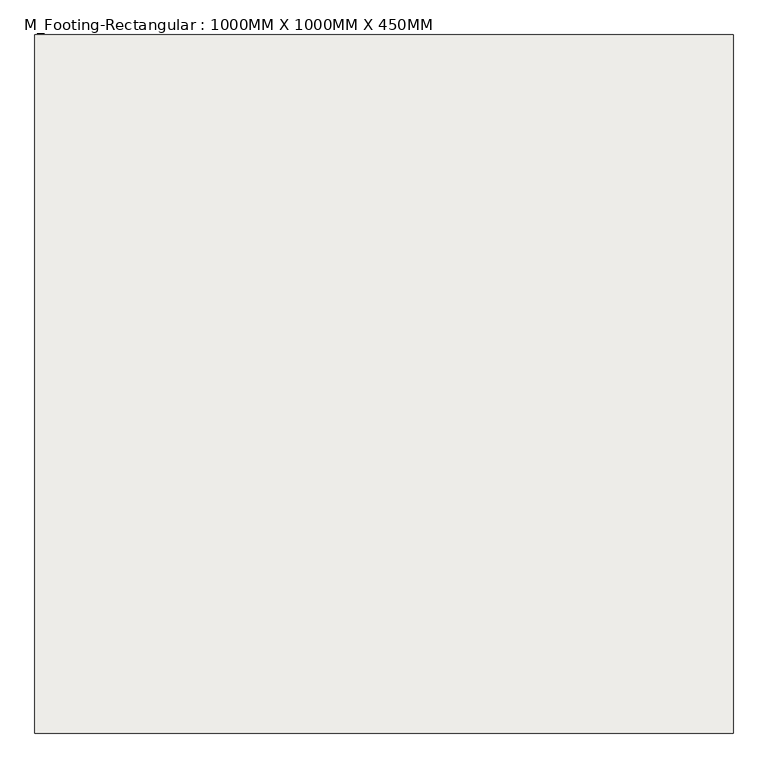
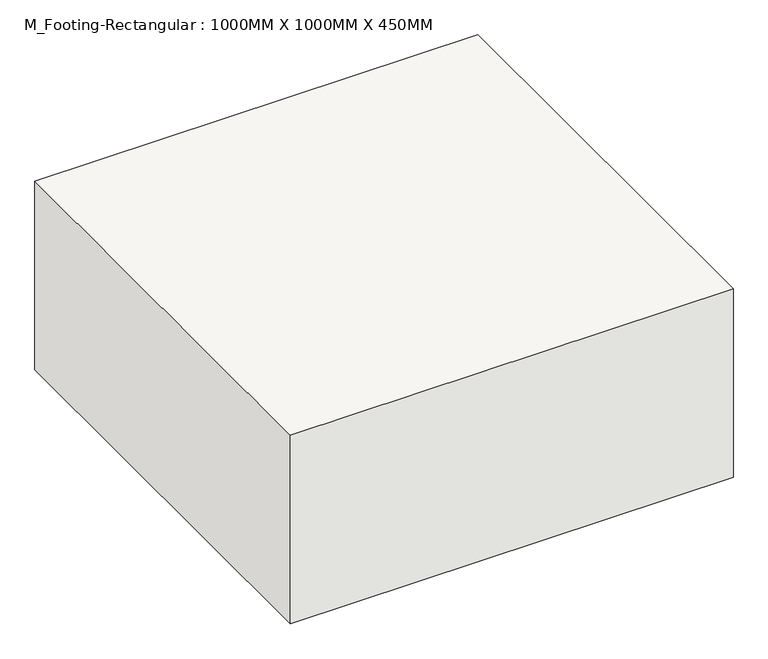
"""IFC4 building model written with IfcOpenShell, lengths in millimetres: slab geometry, M_Footing-Rectangular : 1000MM X 1000MM X 450MM."""

from ifc_helpers import new_model, si_unit, frame, origin, place, context, project, spatial, polyline, outline, extrude, source, transform, mapped, element, save


def m_footing_rectangular_1000mm_x_1000mm_x_450mm_4c97ae35(model_context):
    return source(origin(), model_context, "Body", "SweptSolid", [
        extrude(outline(polyline([(500.0, 500.0), (500.0, -500.0), (-500.0, -500.0), (-500.0, 500.0), (500.0, 500.0)])), frame((0.0, 0.0, -450.0), z_axis=(0.0, 0.0, 1.0), x_axis=(1.0, 0.0, 0.0)), (0.0, 0.0, 1.0), 450.0),
    ])


if __name__ == "__main__":
    model = new_model("IFC4")
    model_context = context("Model", 3, world=origin())
    ifc_project = project(units=[si_unit("LENGTHUNIT", "METRE", prefix="MILLI")], contexts=[model_context])
    site = spatial("IfcSite", under=ifc_project)
    building = spatial("IfcBuilding", under=site)
    placement = place(None, origin())
    m_footing_rectangular_1000mm_x_1000mm_x_450mm_shape = m_footing_rectangular_1000mm_x_1000mm_x_450mm_4c97ae35(model_context)
    element("IfcSlab", 1, ObjectType="M_Footing-Rectangular : 1000MM X 1000MM X 450MM", at=placement, inside=building, context=model_context, shape_type="MappedRepresentation", body=[
        mapped(m_footing_rectangular_1000mm_x_1000mm_x_450mm_shape, transform((0.0, 0.0, 0.0), x_axis=(1.0, 0.0, 0.0), y_axis=(0.0, 1.0, 0.0), z_axis=(0.0, 0.0, 1.0))),
    ])
    save(model, "model.ifc")

# Revit data of these elements
# Type "M_Footing-Rectangular : 1000MM X 1000MM X 450MM"
#   Width = 1000 mm
#   Length = 1000 mm
#   Foundation Thickness = 450 mm
#   Structural Material [instance default] = Concrete, Cast-in-Place gray
#   Assembly Code = ""
# Element 1 (IfcSlab, "M_Footing-Rectangular : 1000MM X 1000MM X 450MM")
#   Materials on its faces: "Concrete, Cast-in-Place gray"
# Materials
#   "Concrete, Cast-in-Place gray": class "Concrete", colour RGB 192 192 192, transparency 0, Description = "Cast-in-place concrete", Cost = 0
